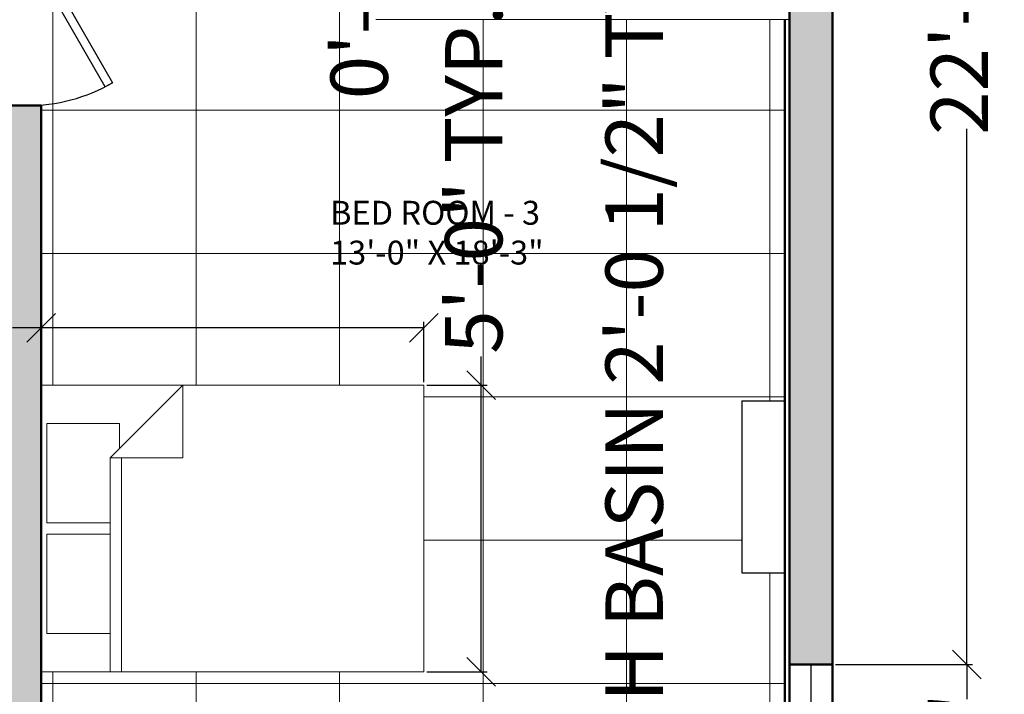
# Model space of a CAD drawing. Units: inches. Extents: x 2371 to 3019, y 129 to 700.
# Tile 11 of 14: x 2753 to 2959, y 358 to 499. Entities that reach past the tile are written whole.
import ezdxf

# ---------------------------------------------------------------- set-up
doc = ezdxf.new("R2010")
doc.units = ezdxf.units.IN
for name, color, linetype, lineweight in [('A-ANNO-DIMS', 2, 'Continuous', 18), ('A-AREA-IDEN', 7, 'Continuous', 25), ('A-DOOR', 4, 'Continuous', 25), ('A-FLOR-PATT', 252, 'Continuous', 13), ('A-FURN', 8, 'Continuous', 18), ('A-GLAZ', 4, 'Continuous', 25), ('A-WALL', 7, 'Continuous', 50), ('A-WALL-PATT', 8, 'Continuous', 13)]:
    doc.layers.add(name, color=color, linetype=linetype, lineweight=lineweight)
doc.styles.get("Standard").update_dxf_attribs({"font": 'arial.ttf'})
doc.dimstyles.new('ISO-25', dxfattribs={"dimtxt": 12, "dimasz": 6, "dimexe": 1.25, "dimexo": 0.625, "dimtad": 0, "dimdec": 1, "dimlunit": 3, "dimtxsty": 'Standard', "dimblk": 'OBLIQUE', "dimblk1": 'ORIGIN2', "dimblk2": 'OBLIQUE', "dimcen": 2.5, "dimadec": 0, "dimazin": 0, "dimtfac": 1, "dimtdec": 1, "dimtmove": 0, "dimatfit": 3, "dimldrblk": 'OBLIQUE', "dimfxl": 1, "dimarcsym": 0})

# ---------------------------------------------------------------- blocks, each defined once
blk = doc.blocks.new('Bed - Queen')
for p, q in [((0, -80.00003), (0, 0)), ((0, 0), (59.99999, 0)), ((59.99999, 0), (59.99999, -80.00003)), ((7.99999, -1.2), (28.79998, -1.2)), ((7.99999, -14.4), (7.99999, -1.2)), ((28.79998, -1.2), (28.79998, -14.4)), ((31.19999, -1.2), (51.99999, -1.2)), ((31.19999, -14.4), (31.19999, -1.2)), ((51.99999, -1.2), (51.99999, -16.4)), ((0, -14.4), (44.8, -14.4)), ((59.99999, -29.6), (44.8, -14.4)), ((44.8, -14.4), (44.8, -29.6)), ((51.99999, -16.4), (46.79936, -16.4)), ((44.8, -16.8), (0, -16.8)), ((44.8, -29.6), (59.99999, -29.6)), ((59.99999, -80.00003), (0, -80.00003))]:
    blk.add_line(p, q)
blk = doc.blocks.new('*U10')
for p, q in [((0, 0), (0, -6)), ((36, 0), (36, -6))]:
    blk.add_line(p, q)
blk.add_lwpolyline([(0, 0), (31.18, 18), (32.05, 16.48), (0.87, -1.52)], close=True)
blk.add_arc((0, 0), 36, 0, 30)
blk = doc.blocks.new('_Oblique')
at = {"color": 0, "linetype": 'ByBlock', "lineweight": -2}
blk.add_line((-0.5, -0.5), (0.5, 0.5), dxfattribs=at)
blk = doc.blocks.new('*D24')
at = {"layer": 'A-ANNO-DIMS', "color": 0, "lineweight": -2, "transparency": 16777216}
for p, q in [((2757.61, 423.1), (2757.61, 435.73)), ((2837.61, 423.1), (2837.61, 435.73)), ((2757.61, 434.48), (2751.61, 434.48)), ((2837.61, 434.48), (2757.61, 434.48))]:
    blk.add_line(p, q, dxfattribs=at)
at = {"layer": 'Defpoints', "color": 0, "lineweight": 25, "transparency": 16777216}
for p in [(2757.61, 434.48), (2757.61, 422.48), (2837.61, 422.48)]:
    blk.add_point(p, dxfattribs=at)
at = {"layer": 'A-ANNO-DIMS', "color": 0, "lineweight": -2, "transparency": 16777216, "xscale": 6, "yscale": 6, "zscale": 6, "rotation": 180}
blk.add_blockref('_Oblique', (2757.61, 434.48), dxfattribs=at)
at = {"layer": 'A-ANNO-DIMS', "color": 0, "lineweight": -2, "transparency": 16777216, "xscale": 6, "yscale": 6, "zscale": 6}
blk.add_blockref('_Oblique', (2837.61, 434.48), dxfattribs=at)
at = {"layer": 'A-ANNO-DIMS', "color": 0, "transparency": 16777216, "insert": (2662.72, 434.48), "char_height": 12, "attachment_point": 5}
blk.add_mtext('QUEEN BED 6\'-8" TYP.', dxfattribs=at)
blk = doc.blocks.new('_Origin2')
at = {"color": 0, "linetype": 'ByBlock', "lineweight": -2}
blk.add_line((-0.5, 0), (-1, 0), dxfattribs=at)
for radius in [0.5, 0.25]:
    blk.add_circle((0, 0), radius, dxfattribs=at)
blk = doc.blocks.new('*D25')
at = {"layer": 'A-ANNO-DIMS', "color": 0, "lineweight": -2, "transparency": 16777216}
for p, q in [((2849.61, 422.48), (2849.61, 428.48)), ((2838.23, 422.48), (2850.86, 422.48)), ((2849.61, 362.48), (2849.61, 422.48)), ((2838.23, 362.48), (2850.86, 362.48))]:
    blk.add_line(p, q, dxfattribs=at)
at = {"layer": 'Defpoints', "color": 0, "lineweight": 25, "transparency": 16777216}
for p in [(2837.61, 422.48), (2849.61, 422.48), (2837.61, 362.48)]:
    blk.add_point(p, dxfattribs=at)
at = {"layer": 'A-ANNO-DIMS', "color": 0, "lineweight": -2, "transparency": 16777216, "xscale": 6, "yscale": 6, "zscale": 6}
for p, rotation in [((2849.61, 422.48), 90), ((2849.61, 362.48), 270)]:
    blk.add_blockref('_Oblique', p, dxfattribs=dict(at, rotation=rotation))
at = {"layer": 'A-ANNO-DIMS', "color": 0, "transparency": 16777216, "insert": (2849.61, 465.67), "char_height": 12, "attachment_point": 5, "rotation": 90}
blk.add_mtext('5\'-0" TYP.', dxfattribs=at)
blk = doc.blocks.new('*D26')
at = {"layer": 'A-ANNO-DIMS', "color": 0, "lineweight": -2, "transparency": 16777216}
for p, q in [((2886.23, 560.02), (2881.92, 560.02)), ((2883.17, 560.02), (2883.17, 535.47)), ((2886.23, 535.47), (2881.92, 535.47)), ((2883.17, 535.47), (2883.17, 529.47))]:
    blk.add_line(p, q, dxfattribs=at)
at = {"layer": 'Defpoints', "color": 0, "lineweight": 25, "transparency": 16777216}
for p in [(2886.85, 560.02), (2883.17, 535.47), (2886.85, 535.47)]:
    blk.add_point(p, dxfattribs=at)
at = {"layer": 'A-ANNO-DIMS', "color": 0, "lineweight": -2, "transparency": 16777216, "xscale": 6, "yscale": 6, "zscale": 6}
for p, rotation in [((2883.17, 560.02), 90), ((2883.17, 535.47), 270)]:
    blk.add_blockref('_Oblique', p, dxfattribs=dict(at, rotation=rotation))
at = {"layer": 'A-ANNO-DIMS', "color": 0, "transparency": 16777216, "insert": (2883.17, 423.09), "char_height": 12, "attachment_point": 5, "rotation": 90}
blk.add_mtext('WASH BASIN 2\'-0 1/2" TYP.', dxfattribs=at)
blk = doc.blocks.new('*D62')
at = {"layer": 'A-ANNO-DIMS', "color": 0, "lineweight": -2, "transparency": 16777216}
for p, q in [((2923.73, 363.98), (2952.41, 363.98)), ((2951.16, 363.98), (2951.16, 356.79)), ((2951.16, 315.98), (2951.16, 323.16)), ((2923.73, 315.98), (2952.41, 315.98))]:
    blk.add_line(p, q, dxfattribs=at)
at = {"layer": 'Defpoints', "color": 0, "lineweight": 25, "transparency": 16777216}
for p in [(2923.11, 363.98), (2951.16, 363.98), (2923.11, 315.98)]:
    blk.add_point(p, dxfattribs=at)
at = {"layer": 'A-ANNO-DIMS', "color": 0, "lineweight": -2, "transparency": 16777216, "xscale": 6, "yscale": 6, "zscale": 6}
for p, rotation in [((2951.16, 363.98), 90), ((2951.16, 315.98), 270)]:
    blk.add_blockref('_Oblique', p, dxfattribs=dict(at, rotation=rotation))
at = {"layer": 'A-ANNO-DIMS', "color": 0, "transparency": 16777216, "insert": (2951.16, 339.98), "char_height": 12, "attachment_point": 5, "rotation": 90}
blk.add_mtext('4\'-0"', dxfattribs=at)
blk = doc.blocks.new('*D63')
at = {"layer": 'A-ANNO-DIMS', "color": 0, "lineweight": -2, "transparency": 16777216}
for p, q in [((2923.73, 630.98), (2952.41, 630.98)), ((2951.16, 630.98), (2951.16, 518.81)), ((2951.16, 363.98), (2951.16, 476.14)), ((2923.73, 363.98), (2952.41, 363.98))]:
    blk.add_line(p, q, dxfattribs=at)
at = {"layer": 'Defpoints', "color": 0, "lineweight": 25, "transparency": 16777216}
for p in [(2923.11, 630.98), (2951.16, 630.98), (2923.11, 363.98)]:
    blk.add_point(p, dxfattribs=at)
at = {"layer": 'A-ANNO-DIMS', "color": 0, "lineweight": -2, "transparency": 16777216, "xscale": 6, "yscale": 6, "zscale": 6}
for p, rotation in [((2951.16, 630.98), 90), ((2951.16, 363.98), 270)]:
    blk.add_blockref('_Oblique', p, dxfattribs=dict(at, rotation=rotation))
at = {"layer": 'A-ANNO-DIMS', "color": 0, "transparency": 16777216, "insert": (2951.16, 497.48), "char_height": 12, "attachment_point": 5, "rotation": 90}
blk.add_mtext('22\'-3"', dxfattribs=at)
blk = doc.blocks.new('*D64')
at = {"layer": 'A-ANNO-DIMS', "color": 0, "lineweight": -2, "transparency": 16777216}
for p, q in [((2798.23, 531.98), (2826.91, 531.98)), ((2825.66, 531.98), (2825.66, 522.98)), ((2798.23, 522.98), (2826.91, 522.98)), ((2825.66, 522.98), (2825.66, 516.98))]:
    blk.add_line(p, q, dxfattribs=at)
at = {"layer": 'Defpoints', "color": 0, "lineweight": 25, "transparency": 16777216}
for p in [(2797.61, 531.98), (2797.61, 522.98), (2825.66, 522.98)]:
    blk.add_point(p, dxfattribs=at)
at = {"layer": 'A-ANNO-DIMS', "color": 0, "lineweight": -2, "transparency": 16777216, "xscale": 6, "yscale": 6, "zscale": 6}
for p, rotation in [((2825.66, 531.98), 90), ((2825.66, 522.98), 270)]:
    blk.add_blockref('_Oblique', p, dxfattribs=dict(at, rotation=rotation))
at = {"layer": 'A-ANNO-DIMS', "color": 0, "transparency": 16777216, "insert": (2825.66, 500.4), "char_height": 12, "attachment_point": 5, "rotation": 90}
blk.add_mtext('0\'-9"', dxfattribs=at)

msp = doc.modelspace()

# ---------------------------------------------------------------- hatches: boundary and pattern name
at = {"layer": 'A-FLOR-PATT'}
h = msp.add_hatch(dxfattribs=at)
h.set_pattern_fill('_USER', color=256, scale=30, pattern_type=0)
h.set_pattern_definition([(0, (0, 0), (0, 30), [])])
h.paths.add_polyline_path([(2913.11, 498.98), (2827.61, 498.98), (2827.61, 531.98), (2832.11, 531.98), (2832.11, 537.98), (2833.61, 537.98), (2833.61, 605.98), (2818.35, 605.98, -1), (2796.86, 605.98), (2781.61, 605.98), (2781.61, 603.98), (2781.61, 533.98), (2757.61, 533.98), (2757.61, 531.98), (2797.61, 531.98), (2797.61, 522.98), (2757.61, 522.98), (2757.61, 516.98), (2754.59, 516.98), (2772.52, 485.76), (2771.01, 484.89), (2770.98, 484.93, -0.097552), (2757.61, 481.1), (2757.61, 422.48), (2837.61, 422.48), (2837.61, 362.48), (2757.61, 362.48), (2757.61, 303.98), (2835.86, 303.98, -0.09439), (2793.86, 311.98), (2793.86, 337.98), (2799.86, 337.98), (2799.86, 336.42), (2871.86, 336.42), (2871.86, 337.98), (2877.86, 337.98), (2877.86, 311.98, -0.09439), (2835.86, 303.98), (2913.11, 303.98), (2913.11, 383.18), (2904.11, 383.18), (2904.11, 419.18), (2913.11, 419.18)])
h.paths.add_polyline_path([(2788.88, 332.88), (2788.88, 308.88), (2764.88, 308.88), (2764.88, 332.88)], flags=16)
h.paths.add_polyline_path([(2788.4, 325.04, -1), (2774.4, 325.04, -1)], flags=0)
h.paths.add_polyline_path([(2781.4, 328.04), (2784.4, 325.04), (2781.4, 322.04), (2778.4, 325.04)], flags=0)
h.paths.add_polyline_path([(2782.4, 325.04, -1), (2780.4, 325.04, -1)], flags=0)
h.paths.add_polyline_path([(2748.61, 480.99), (2754.51, 480.98, 0.119303), (2770.98, 484.93), (2753.07, 516.1), (2754.59, 516.98), (2748.61, 516.98), (2748.61, 539.98), (2712.61, 539.98), (2665.11, 539.98, -0.09439), (2707.11, 531.98), (2707.11, 505.98), (2701.11, 505.98), (2701.11, 507.53), (2629.11, 507.53), (2629.11, 505.98), (2623.11, 505.98), (2623.11, 531.98, -0.09439), (2665.11, 539.98), (2581.61, 539.98), (2581.61, 522.98), (2581.61, 477.98, -0.131044), (2589.61, 507.98), (2615.61, 507.98), (2615.61, 501.98), (2614.05, 501.98), (2614.05, 453.98), (2615.61, 453.98), (2615.61, 447.98), (2589.61, 447.98, -0.131044), (2581.61, 477.98), (2581.61, 432.98), (2572.61, 432.98, 0.119303), (2556.14, 428.99), (2574.12, 397.85), (2572.61, 396.98), (2578.61, 396.98), (2581.61, 396.98), (2581.61, 390.98), (2748.61, 390.98)])
h.paths.add_polyline_path([(2683.1, 447.25), (2652.43, 447.25), (2652.43, 492.22), (2683.1, 492.22)], flags=16)
h.paths.add_polyline_path([(2682.1, 448.25), (2653.43, 448.25), (2653.43, 491.22), (2682.1, 491.22)], flags=0)
h.paths.add_polyline_path([(2613.58, 512.06), (2589.58, 512.06), (2589.58, 536.06), (2613.58, 536.06)], flags=16)
h.paths.add_polyline_path([(2599.1, 528.22, -1), (2613.1, 528.22, -1)], flags=0)
h.paths.add_polyline_path([(2609.1, 528.22), (2606.1, 525.22), (2603.1, 528.22), (2606.1, 531.22)], flags=0)
h.paths.add_polyline_path([(2607.1, 528.22, -1), (2605.1, 528.22, -1)], flags=0)
h.paths.add_polyline_path([(2581.61, 522.98), (2581.61, 621.98), (2572.61, 621.98), (2572.61, 522.98), (2572.61, 500.98), (2565.85, 500.98), (2565.85, 500.15), (2564.82, 500.15), (2561.16, 500.19), (2561.16, 500.17), (2560.13, 500.3), (2560.22, 500.98), (2556.38, 500.98), (2556.43, 500.22), (2555.4, 500.14), (2555.34, 500.98), (2551.07, 500.98), (2551.07, 500.15), (2550.04, 500.15), (2547.64, 500.19), (2547.64, 500.15), (2546.61, 500.15), (2541.79, 500.22), (2540.72, 500.13), (2540.65, 500.98), (2533.37, 500.98), (2533.37, 500.15), (2532.34, 500.15), (2529.13, 500.21), (2529.12, 500.13), (2528.09, 500.22), (2528.16, 500.98), (2523.23, 500.98), (2523.23, 500.15), (2522.2, 500.15), (2519.8, 500.21), (2519.8, 500.15), (2518.77, 500.15), (2514.45, 500.26), (2514.44, 500.14), (2513.41, 500.22), (2513.47, 500.98), (2509.62, 500.98), (2509.71, 500.3), (2508.69, 500.17), (2508.58, 500.98), (2505.03, 500.98), (2505.03, 500.15), (2503.99, 500.15), (2501.07, 500.29), (2501.07, 500.15), (2500.04, 500.15), (2496.44, 500.37), (2496.44, 500.15), (2495.4, 500.15), (2492.55, 500.41), (2492.18, 500.35), (2492.09, 500.98), (2486.11, 500.98), (2486.11, 524.98), (2486.11, 531.98), (2490.61, 531.98), (2490.61, 537.98), (2492.11, 537.98), (2492.11, 605.98), (2476.85, 605.98, -1), (2455.36, 605.98), (2440.11, 605.98), (2440.11, 533.98), (2416.11, 533.98), (2416.11, 605.98), (2416.11, 621.98), (2536.61, 621.98), (2536.61, 630.98), (2407.11, 630.98), (2407.11, 363.98), (2416.11, 363.98), (2416.11, 431.48), (2496.11, 431.48), (2496.11, 371.48), (2416.11, 371.48), (2416.11, 303.98), (2494.36, 303.98, -0.09439), (2452.36, 311.98), (2452.36, 337.98), (2458.36, 337.98), (2458.36, 336.42), (2530.36, 336.42), (2530.36, 337.98), (2536.36, 337.98), (2536.36, 311.98, -0.09439), (2494.36, 303.98), (2572.61, 303.98), (2572.61, 381.98), (2572.61, 396.98), (2554.61, 428.15), (2556.12, 429.03), (2556.14, 428.99, -0.119303), (2572.61, 432.98), (2578.61, 432.98), (2581.61, 432.98)])
h.paths.add_polyline_path([(2450.11, 500.98), (2444.5, 500.98), (2444.44, 500.14), (2443.41, 500.22), (2443.47, 500.98), (2439.62, 500.98), (2439.71, 500.3), (2438.69, 500.17), (2438.58, 500.98), (2435.02, 500.98), (2435.02, 500.15), (2433.99, 500.15), (2433.99, 500.98), (2431.07, 500.98), (2431.07, 500.15), (2430.04, 500.15), (2430.04, 500.98), (2426.43, 500.98), (2426.43, 500.15), (2425.4, 500.15), (2425.4, 500.98), (2423.13, 500.98), (2423.2, 500.5), (2422.18, 500.35), (2422.09, 500.98), (2416.11, 500.98), (2416.11, 524.98), (2416.11, 531.98), (2450.11, 531.98), (2450.11, 522.98)], flags=16)
h.paths.add_polyline_path([(2449.11, 501.98), (2417.11, 501.98), (2417.11, 522.98), (2417.11, 523.98), (2449.11, 523.98)], flags=0)
h.paths.add_polyline_path([(2420.7, 510.73), (2419.36, 520.07), (2420.38, 520.22), (2421.74, 510.73), (2425.4, 510.73), (2425.4, 520.07), (2426.43, 520.07), (2426.43, 510.73), (2430.04, 510.73), (2430.04, 520.07), (2431.07, 520.07), (2431.07, 510.73), (2433.99, 510.73), (2433.99, 520.07), (2435.02, 520.07), (2435.02, 510.73), (2437.35, 510.73), (2436.18, 519.93), (2437.2, 520.06), (2438.39, 510.73), (2444.17, 510.73), (2444.85, 520.08), (2445.88, 520.01), (2445.21, 510.73)], flags=0)
h.paths.add_polyline_path([(2446.94, 336.11), (2446.94, 312.11), (2422.94, 312.11), (2422.94, 336.11)], flags=16)
h.paths.add_polyline_path([(2446.46, 328.27, -1), (2432.46, 328.27, -1)], flags=0)
h.paths.add_polyline_path([(2439.46, 331.27), (2442.46, 328.27), (2439.46, 325.27), (2436.46, 328.27)], flags=0)
h.paths.add_polyline_path([(2440.46, 328.27, -1), (2438.46, 328.27, -1)], flags=0)
h.paths.add_polyline_path([(2816, 444.88), (2866.87, 444.88), (2866.87, 463.54), (2816, 463.54)], flags=24)
h.paths.add_polyline_path([(2794.21, 558.3), (2833.34, 558.3), (2833.34, 576.96), (2794.21, 576.96)], flags=24)
h.paths.add_polyline_path([(2651.69, 411.53), (2711.04, 411.53), (2711.04, 430.19), (2651.69, 430.19)], flags=24)
h.paths.add_polyline_path([(2494.09, 444.88), (2544.97, 444.88), (2544.97, 463.54), (2494.09, 463.54)], flags=24)
h.paths.add_polyline_path([(2444.55, 565.02), (2483.69, 565.02), (2483.69, 583.68), (2444.55, 583.68)], flags=24)
h = msp.add_hatch(dxfattribs=at)
h.set_pattern_fill('_USER', color=256, scale=30, angle=90, pattern_type=0)
h.set_pattern_definition([(90, (0, 0), (-30, 2e-15), [])])
h.paths.add_polyline_path([(2913.11, 498.98), (2827.61, 498.98), (2827.61, 531.98), (2832.11, 531.98), (2832.11, 537.98), (2833.61, 537.98), (2833.61, 605.98), (2818.35, 605.98, -1), (2796.86, 605.98), (2781.61, 605.98), (2781.61, 603.98), (2781.61, 533.98), (2757.61, 533.98), (2757.61, 531.98), (2797.61, 531.98), (2797.61, 522.98), (2757.61, 522.98), (2757.61, 516.98), (2754.59, 516.98), (2772.52, 485.76), (2771.01, 484.89), (2770.98, 484.93, -0.097552), (2757.61, 481.1), (2757.61, 422.48), (2837.61, 422.48), (2837.61, 362.48), (2757.61, 362.48), (2757.61, 303.98), (2835.86, 303.98, -0.09439), (2793.86, 311.98), (2793.86, 337.98), (2799.86, 337.98), (2799.86, 336.42), (2871.86, 336.42), (2871.86, 337.98), (2877.86, 337.98), (2877.86, 311.98, -0.09439), (2835.86, 303.98), (2913.11, 303.98), (2913.11, 383.18), (2904.11, 383.18), (2904.11, 419.18), (2913.11, 419.18)])
h.paths.add_polyline_path([(2788.88, 332.88), (2788.88, 308.88), (2764.88, 308.88), (2764.88, 332.88)], flags=16)
h.paths.add_polyline_path([(2788.4, 325.04, -1), (2774.4, 325.04, -1)], flags=0)
h.paths.add_polyline_path([(2781.4, 328.04), (2784.4, 325.04), (2781.4, 322.04), (2778.4, 325.04)], flags=0)
h.paths.add_polyline_path([(2782.4, 325.04, -1), (2780.4, 325.04, -1)], flags=0)
h.paths.add_polyline_path([(2748.61, 480.99), (2754.51, 480.98, 0.119303), (2770.98, 484.93), (2753.07, 516.1), (2754.59, 516.98), (2748.61, 516.98), (2748.61, 539.98), (2712.61, 539.98), (2665.11, 539.98, -0.09439), (2707.11, 531.98), (2707.11, 505.98), (2701.11, 505.98), (2701.11, 507.53), (2629.11, 507.53), (2629.11, 505.98), (2623.11, 505.98), (2623.11, 531.98, -0.09439), (2665.11, 539.98), (2581.61, 539.98), (2581.61, 522.98), (2581.61, 477.98, -0.131044), (2589.61, 507.98), (2615.61, 507.98), (2615.61, 501.98), (2614.05, 501.98), (2614.05, 453.98), (2615.61, 453.98), (2615.61, 447.98), (2589.61, 447.98, -0.131044), (2581.61, 477.98), (2581.61, 432.98), (2572.61, 432.98, 0.119303), (2556.14, 428.99), (2574.12, 397.85), (2572.61, 396.98), (2578.61, 396.98), (2581.61, 396.98), (2581.61, 390.98), (2748.61, 390.98)])
h.paths.add_polyline_path([(2683.1, 447.25), (2652.43, 447.25), (2652.43, 492.22), (2683.1, 492.22)], flags=16)
h.paths.add_polyline_path([(2682.1, 448.25), (2653.43, 448.25), (2653.43, 491.22), (2682.1, 491.22)], flags=0)
h.paths.add_polyline_path([(2613.58, 512.06), (2589.58, 512.06), (2589.58, 536.06), (2613.58, 536.06)], flags=16)
h.paths.add_polyline_path([(2599.1, 528.22, -1), (2613.1, 528.22, -1)], flags=0)
h.paths.add_polyline_path([(2609.1, 528.22), (2606.1, 525.22), (2603.1, 528.22), (2606.1, 531.22)], flags=0)
h.paths.add_polyline_path([(2607.1, 528.22, -1), (2605.1, 528.22, -1)], flags=0)
h.paths.add_polyline_path([(2581.61, 522.98), (2581.61, 621.98), (2572.61, 621.98), (2572.61, 522.98), (2572.61, 500.98), (2565.85, 500.98), (2565.85, 500.15), (2564.82, 500.15), (2561.16, 500.19), (2561.16, 500.17), (2560.13, 500.3), (2560.22, 500.98), (2556.38, 500.98), (2556.43, 500.22), (2555.4, 500.14), (2555.34, 500.98), (2551.07, 500.98), (2551.07, 500.15), (2550.04, 500.15), (2547.64, 500.19), (2547.64, 500.15), (2546.61, 500.15), (2541.79, 500.22), (2540.72, 500.13), (2540.65, 500.98), (2533.37, 500.98), (2533.37, 500.15), (2532.34, 500.15), (2529.13, 500.21), (2529.12, 500.13), (2528.09, 500.22), (2528.16, 500.98), (2523.23, 500.98), (2523.23, 500.15), (2522.2, 500.15), (2519.8, 500.21), (2519.8, 500.15), (2518.77, 500.15), (2514.45, 500.26), (2514.44, 500.14), (2513.41, 500.22), (2513.47, 500.98), (2509.62, 500.98), (2509.71, 500.3), (2508.69, 500.17), (2508.58, 500.98), (2505.03, 500.98), (2505.03, 500.15), (2503.99, 500.15), (2501.07, 500.29), (2501.07, 500.15), (2500.04, 500.15), (2496.44, 500.37), (2496.44, 500.15), (2495.4, 500.15), (2492.55, 500.41), (2492.18, 500.35), (2492.09, 500.98), (2486.11, 500.98), (2486.11, 524.98), (2486.11, 531.98), (2490.61, 531.98), (2490.61, 537.98), (2492.11, 537.98), (2492.11, 605.98), (2476.85, 605.98, -1), (2455.36, 605.98), (2440.11, 605.98), (2440.11, 533.98), (2416.11, 533.98), (2416.11, 605.98), (2416.11, 621.98), (2536.61, 621.98), (2536.61, 630.98), (2407.11, 630.98), (2407.11, 363.98), (2416.11, 363.98), (2416.11, 431.48), (2496.11, 431.48), (2496.11, 371.48), (2416.11, 371.48), (2416.11, 303.98), (2494.36, 303.98, -0.09439), (2452.36, 311.98), (2452.36, 337.98), (2458.36, 337.98), (2458.36, 336.42), (2530.36, 336.42), (2530.36, 337.98), (2536.36, 337.98), (2536.36, 311.98, -0.09439), (2494.36, 303.98), (2572.61, 303.98), (2572.61, 381.98), (2572.61, 396.98), (2554.61, 428.15), (2556.12, 429.03), (2556.14, 428.99, -0.119303), (2572.61, 432.98), (2578.61, 432.98), (2581.61, 432.98)])
h.paths.add_polyline_path([(2450.11, 500.98), (2444.5, 500.98), (2444.44, 500.14), (2443.41, 500.22), (2443.47, 500.98), (2439.62, 500.98), (2439.71, 500.3), (2438.69, 500.17), (2438.58, 500.98), (2435.02, 500.98), (2435.02, 500.15), (2433.99, 500.15), (2433.99, 500.98), (2431.07, 500.98), (2431.07, 500.15), (2430.04, 500.15), (2430.04, 500.98), (2426.43, 500.98), (2426.43, 500.15), (2425.4, 500.15), (2425.4, 500.98), (2423.13, 500.98), (2423.2, 500.5), (2422.18, 500.35), (2422.09, 500.98), (2416.11, 500.98), (2416.11, 524.98), (2416.11, 531.98), (2450.11, 531.98), (2450.11, 522.98)], flags=16)
h.paths.add_polyline_path([(2449.11, 501.98), (2417.11, 501.98), (2417.11, 522.98), (2417.11, 523.98), (2449.11, 523.98)], flags=0)
h.paths.add_polyline_path([(2420.7, 510.73), (2419.36, 520.07), (2420.38, 520.22), (2421.74, 510.73), (2425.4, 510.73), (2425.4, 520.07), (2426.43, 520.07), (2426.43, 510.73), (2430.04, 510.73), (2430.04, 520.07), (2431.07, 520.07), (2431.07, 510.73), (2433.99, 510.73), (2433.99, 520.07), (2435.02, 520.07), (2435.02, 510.73), (2437.35, 510.73), (2436.18, 519.93), (2437.2, 520.06), (2438.39, 510.73), (2444.17, 510.73), (2444.85, 520.08), (2445.88, 520.01), (2445.21, 510.73)], flags=0)
h.paths.add_polyline_path([(2446.94, 336.11), (2446.94, 312.11), (2422.94, 312.11), (2422.94, 336.11)], flags=16)
h.paths.add_polyline_path([(2446.46, 328.27, -1), (2432.46, 328.27, -1)], flags=0)
h.paths.add_polyline_path([(2439.46, 331.27), (2442.46, 328.27), (2439.46, 325.27), (2436.46, 328.27)], flags=0)
h.paths.add_polyline_path([(2440.46, 328.27, -1), (2438.46, 328.27, -1)], flags=0)
h.paths.add_polyline_path([(2816, 444.88), (2866.87, 444.88), (2866.87, 463.54), (2816, 463.54)], flags=24)
h.paths.add_polyline_path([(2794.21, 558.3), (2833.34, 558.3), (2833.34, 576.96), (2794.21, 576.96)], flags=24)
h.paths.add_polyline_path([(2651.69, 411.53), (2711.04, 411.53), (2711.04, 430.19), (2651.69, 430.19)], flags=24)
h.paths.add_polyline_path([(2494.09, 444.88), (2544.97, 444.88), (2544.97, 463.54), (2494.09, 463.54)], flags=24)
h.paths.add_polyline_path([(2444.55, 565.02), (2483.69, 565.02), (2483.69, 583.68), (2444.55, 583.68)], flags=24)
at = {"layer": 'A-WALL-PATT'}
h = msp.add_hatch(color=256, dxfattribs=at)
h.dxf.hatch_style = 1
h.paths.add_polyline_path([(2536.61, 630.98), (2407.11, 630.98), (2407.11, 363.98), (2416.11, 363.98), (2416.11, 498.98), (2416.11, 522.98), (2416.11, 531.98), (2416.11, 603.98), (2416.11, 621.98), (2536.61, 621.98)])
h.paths.add_polyline_path([(2630.98, 630.98), (2560.61, 630.98), (2560.61, 621.98), (2630.98, 621.98)])
h.paths.add_polyline_path([(2878.11, 630.98), (2699.23, 630.98), (2699.23, 621.98), (2878.11, 621.98)])
h.paths.add_polyline_path([(2496.61, 621.98), (2492.11, 621.98), (2492.11, 569.98), (2496.61, 569.98)], flags=17)
h.paths.add_polyline_path([(2581.61, 621.98), (2572.61, 621.98), (2572.61, 522.98), (2572.61, 498.98), (2572.61, 432.98), (2578.61, 432.98), (2581.61, 432.98), (2581.61, 522.98)])
h.paths.add_polyline_path([(2572.61, 531.98), (2486.11, 531.98), (2486.11, 522.98), (2572.61, 522.98)])
h.paths.add_polyline_path([(2450.11, 531.98), (2440.11, 531.98), (2416.11, 531.98), (2416.11, 522.98), (2450.11, 522.98)], flags=17)
h.paths.add_polyline_path([(2416.11, 315.98), (2407.11, 315.98), (2407.11, 294.98), (2458.11, 294.98), (2458.11, 303.98), (2416.11, 303.98)])
h.paths.add_polyline_path([(2757.61, 303.98), (2530.61, 303.98), (2530.61, 294.98), (2757.61, 294.98)])
h.paths.add_polyline_path([(2581.61, 381.98), (2605.61, 381.98), (2617.61, 381.98), (2617.61, 390.98), (2581.61, 390.98), (2581.61, 396.98), (2572.61, 396.98), (2572.61, 381.98), (2572.61, 303.98), (2581.61, 303.98)])
h.paths.add_polyline_path([(2757.61, 480.98), (2748.61, 480.98), (2748.61, 381.98), (2748.61, 303.98), (2757.61, 303.98), (2757.61, 381.98), (2757.61, 422.48)])
h.paths.add_polyline_path([(2797.61, 531.98), (2757.61, 531.98), (2757.61, 603.98), (2757.61, 621.98), (2748.61, 621.98), (2748.61, 516.99), (2754.59, 516.98), (2757.61, 516.98), (2757.61, 522.98), (2797.61, 522.98)])
h.paths.add_polyline_path([(2913.11, 531.98), (2827.61, 531.98), (2827.61, 522.98), (2913.11, 522.98)])
h.paths.add_polyline_path([(2923.11, 630.98), (2902.11, 630.98), (2902.11, 621.98), (2914.11, 621.98), (2914.11, 363.98), (2923.11, 363.98)])
h.paths.add_polyline_path([(2923.11, 315.98), (2914.11, 315.98), (2914.11, 303.98), (2866.11, 303.98), (2866.11, 294.98), (2923.11, 294.98)])
h.paths.add_polyline_path([(2793.61, 303.98), (2757.61, 303.98), (2757.61, 294.98), (2793.61, 294.98)])

# ---------------------------------------------------------------- linework, layer by layer
at = {"layer": 'A-FURN'}
msp.add_line((2914.11, 498.98), (2827.61, 498.98), dxfattribs=at)
at = {"layer": 'A-GLAZ'}
for p, q in [((2904.11, 419.18), (2913.11, 419.18)), ((2904.11, 419.18), (2904.11, 383.18)), ((2904.11, 383.18), (2913.11, 383.18)), ((2918.61, 315.98), (2918.61, 363.98))]:
    msp.add_line(p, q, dxfattribs=at)
at = {"layer": 'A-WALL'}
for p, q in [((2923.11, 294.98), (2923.11, 630.98)), ((2914.11, 303.98), (2914.11, 621.98)), ((2913.11, 303.98), (2913.11, 498.98)), ((2757.61, 480.98), (2748.61, 480.98)), ((2757.61, 381.98), (2757.61, 480.98)), ((2757.61, 303.98), (2757.61, 381.98)), ((2914.11, 363.98), (2923.11, 363.98))]:
    msp.add_line(p, q, dxfattribs=at)

# ---------------------------------------------------------------- block references
at = {"layer": 'A-DOOR', "rotation": 269.8782938999684}
msp.add_blockref('*U10', (2754.59, 516.98), dxfattribs=at)
at = {"layer": 'A-FURN', "rotation": 90}
msp.add_blockref('Bed - Queen', (2757.61, 362.48), dxfattribs=at)

# ---------------------------------------------------------------- texts
at = {"layer": 'A-AREA-IDEN', "ltscale": 2, "insert": (2818.01, 461.06), "char_height": 5, "attachment_point": 1}
msp.add_mtext_dynamic_manual_height_columns('BED ROOM - 3\\P13\'-0" X 18\'-3"', width=49.6634, gutter_width=12.5, heights=[0], dxfattribs=at)

# ---------------------------------------------------------------- dimensions: what is measured, and where the dimension line sits
at = {"layer": 'A-ANNO-DIMS'}
for base, p1, p2, angle, picture, middle in [((2951.16, 630.98), (2923.11, 363.98), (2923.11, 630.98), 90, '*D63', (2951.16, 497.48)), ((2825.66, 522.98), (2797.61, 531.98), (2797.61, 522.98), 270, '*D64', (2825.66, 500.4)), ((2951.16, 363.98), (2923.11, 315.98), (2923.11, 363.98), 90, '*D62', (2951.16, 339.98))]:
    dim = msp.add_linear_dim(base=base, p1=p1, p2=p2, angle=angle, dimstyle='ISO-25', override={"dimdec": 1, "dimlfac": 1, "dimrnd": 0, "dimzin": 1, "dimdsep": 46, "dimlunit": 4, "dimfrac": 2}, dxfattribs=at)
    dim.commit()
    dim.dimension.update_dxf_attribs({"geometry": picture, "text_midpoint": middle})
for base, p1, p2, angle, text, picture, middle in [((2883.1676, 535.4732), (2886.8502, 560.0241), (2886.8502, 535.4732), 270, 'WASH BASIN <> TYP.', '*D26', (2883.1676, 423.0911)), ((2849.61, 422.48), (2837.61, 362.48), (2837.61, 422.48), 90, '<> TYP.', '*D25', (2849.61, 465.67)), ((2757.61, 434.48), (2837.61, 422.48), (2757.61, 422.48), 180, 'QUEEN BED <> TYP.', '*D24', (2662.72, 434.48))]:
    dim = msp.add_linear_dim(base=base, p1=p1, p2=p2, angle=angle, text=text, dimstyle='ISO-25', override={"dimdec": 1, "dimrnd": 0, "dimzin": 1, "dimlunit": 4, "dimfrac": 2}, dxfattribs=at)
    dim.commit()
    dim.dimension.update_dxf_attribs({"geometry": picture, "text_midpoint": middle})

doc.saveas('drawing.dxf')
